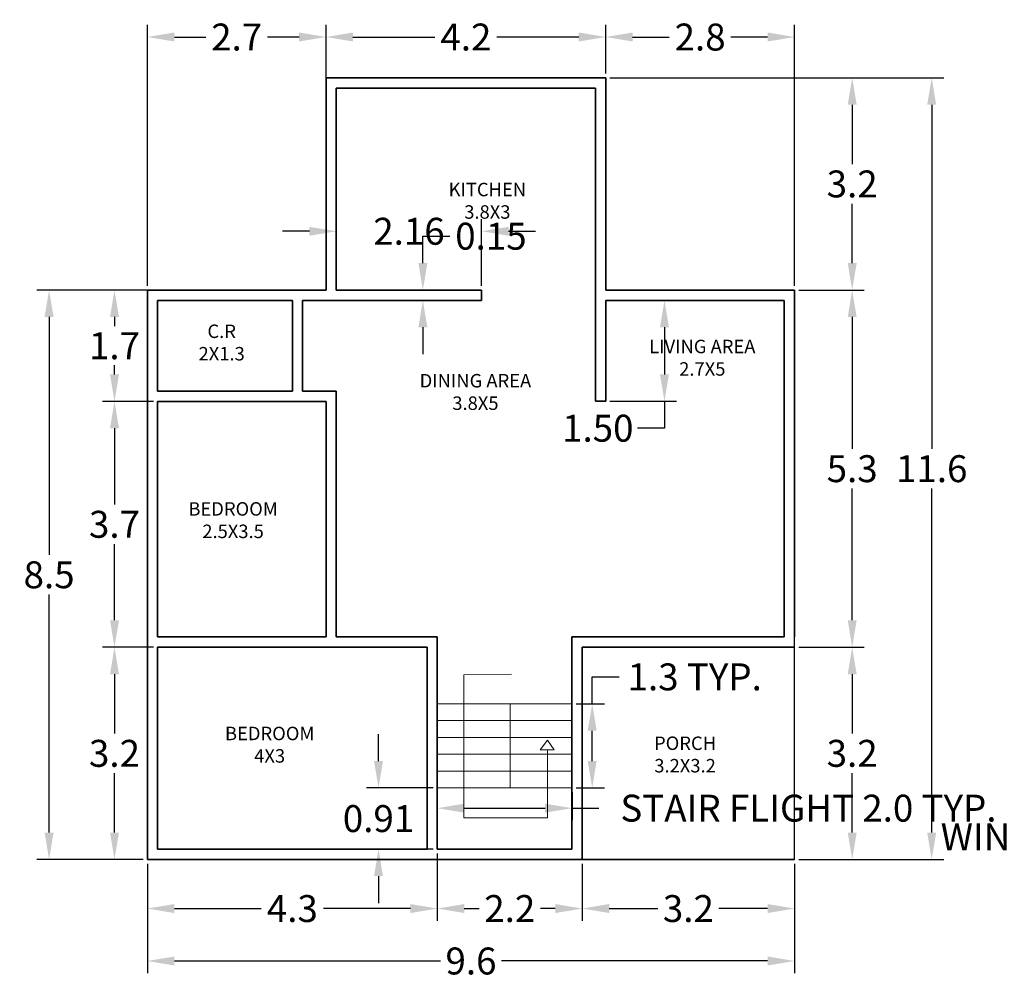
# Model space of a CAD drawing. Units: metres. Extents: x 24.2 to 58.5, y -14.5 to 15.2.
# Tile 2 of 7: x 24.2 to 38.9, y 0.1 to 14.4. Entities that reach past the tile are written whole.
import ezdxf

# ---------------------------------------------------------------- set-up
doc = ezdxf.new("R2010")
doc.units = ezdxf.units.M
doc.header["$MEASUREMENT"] = 0
for name, color, linetype, lineweight in [('A-ANNO-SYMB', 90, 'Continuous', 18), ('A-AREA-IDEN', 1, 'Continuous', 18), ('A-FLOR', 7, 'Continuous', 25), ('A-FLOR-STRS', 7, 'Continuous', 18), ('A-WALL', 7, 'Continuous', 35), ('DIMENSION', 90, 'Continuous', 18)]:
    doc.layers.add(name, color=color, linetype=linetype, lineweight=lineweight)
doc.styles.get("Standard").update_dxf_attribs({"font": 'arial.ttf'})
doc.dimstyles.get("Standard").update_dxf_attribs({"dimtxt": 0.4, "dimasz": 0.4, "dimexe": 0.18, "dimexo": 0.0625, "dimgap": 0.09, "dimtad": 0, "dimtih": 1, "dimtoh": 1, "dimdec": 1, "dimzin": 0, "dimdsep": 46, "dimtxsty": 'Standard', "dimcen": 0.09, "dimadec": 0, "dimazin": 0, "dimtfac": 1, "dimtdec": 1, "dimtofl": 0, "dimtmove": 0, "dimatfit": 3, "dimfxl": 1, "dimtolj": 1, "dimtzin": 0, "dimarcsym": 0})

# ---------------------------------------------------------------- blocks, each defined once
blk = doc.blocks.new('*D1')
at = {"layer": 'Defpoints', "color": 0, "transparency": 16777216}
for p in [(30.434, 2.049), (26.129, 1.896), (30.434, 1.168)]:
    blk.add_point(p, dxfattribs=at)
at = {"layer": 'DIMENSION', "color": 0, "lineweight": -2, "transparency": 16777216}
for p, q in [((30.434, 1.986), (30.434, 0.988)), ((26.129, 1.834), (26.129, 0.988)), ((26.529, 1.168), (27.819, 1.168)), ((30.034, 1.168), (28.744, 1.168))]:
    blk.add_line(p, q, dxfattribs=at)
at = {"layer": 'DIMENSION', "color": 0, "transparency": 16777216}
for points in [[(26.529, 1.235), (26.529, 1.101), (26.129, 1.168)], [(30.034, 1.235), (30.034, 1.101), (30.434, 1.168)]]:
    blk.add_solid(points, dxfattribs=at)
at = {"layer": 'DIMENSION', "color": 0, "transparency": 16777216, "insert": (28.281, 1.168), "char_height": 0.4, "attachment_point": 5}
blk.add_mtext('\\A1;4.3', dxfattribs=at)
blk = doc.blocks.new('*D2')
at = {"layer": 'Defpoints', "color": 0, "transparency": 16777216}
for p in [(30.434, 2.049), (32.586, 1.896), (32.586, 1.168)]:
    blk.add_point(p, dxfattribs=at)
at = {"layer": 'DIMENSION', "color": 0, "lineweight": -2, "transparency": 16777216}
for p, q in [((30.434, 1.986), (30.434, 0.988)), ((32.586, 1.834), (32.586, 0.988)), ((30.834, 1.168), (31.054, 1.168)), ((32.186, 1.168), (31.965, 1.168))]:
    blk.add_line(p, q, dxfattribs=at)
at = {"layer": 'DIMENSION', "color": 0, "transparency": 16777216}
for points in [[(30.834, 1.235), (30.834, 1.101), (30.434, 1.168)], [(32.186, 1.235), (32.186, 1.101), (32.586, 1.168)]]:
    blk.add_solid(points, dxfattribs=at)
at = {"layer": 'DIMENSION', "color": 0, "transparency": 16777216, "insert": (31.51, 1.168), "char_height": 0.4, "attachment_point": 5}
blk.add_mtext('\\A1;2.2', dxfattribs=at)
blk = doc.blocks.new('*D3')
at = {"layer": 'Defpoints', "color": 0, "transparency": 16777216}
for p in [(32.586, 1.896), (35.739, 1.896), (35.739, 1.168)]:
    blk.add_point(p, dxfattribs=at)
at = {"layer": 'DIMENSION', "color": 0, "lineweight": -2, "transparency": 16777216}
for p, q in [((32.586, 1.834), (32.586, 0.988)), ((35.739, 1.834), (35.739, 0.988)), ((32.986, 1.168), (33.71, 1.168)), ((35.339, 1.168), (34.614, 1.168))]:
    blk.add_line(p, q, dxfattribs=at)
at = {"layer": 'DIMENSION', "color": 0, "transparency": 16777216}
for points in [[(32.986, 1.235), (32.986, 1.101), (32.586, 1.168)], [(35.339, 1.235), (35.339, 1.101), (35.739, 1.168)]]:
    blk.add_solid(points, dxfattribs=at)
at = {"layer": 'DIMENSION', "color": 0, "transparency": 16777216, "insert": (34.162, 1.168), "char_height": 0.4, "attachment_point": 5}
blk.add_mtext('\\A1;3.2', dxfattribs=at)
blk = doc.blocks.new('*D4')
at = {"layer": 'Defpoints', "color": 0, "transparency": 16777216}
for p in [(25.64, 5.049), (26.281, 5.049), (26.129, 1.896)]:
    blk.add_point(p, dxfattribs=at)
at = {"layer": 'DIMENSION', "color": 0, "lineweight": -2, "transparency": 16777216}
for p, q in [((26.219, 5.049), (25.46, 5.049)), ((25.64, 4.649), (25.64, 3.767)), ((25.64, 2.296), (25.64, 3.178)), ((26.066, 1.896), (25.46, 1.896))]:
    blk.add_line(p, q, dxfattribs=at)
at = {"layer": 'DIMENSION', "color": 0, "transparency": 16777216}
for points in [[(25.574, 4.649), (25.707, 4.649), (25.64, 5.049)], [(25.574, 2.296), (25.707, 2.296), (25.64, 1.896)]]:
    blk.add_solid(points, dxfattribs=at)
at = {"layer": 'DIMENSION', "color": 0, "transparency": 16777216, "insert": (25.64, 3.473), "char_height": 0.4, "attachment_point": 5}
blk.add_mtext('\\A1;3.2', dxfattribs=at)
blk = doc.blocks.new('*D5')
at = {"layer": 'Defpoints', "color": 0, "transparency": 16777216}
for p in [(25.64, 8.701), (26.281, 8.701), (26.281, 5.049)]:
    blk.add_point(p, dxfattribs=at)
at = {"layer": 'DIMENSION', "color": 0, "lineweight": -2, "transparency": 16777216}
for p, q in [((26.219, 8.701), (25.46, 8.701)), ((25.64, 8.301), (25.64, 7.169)), ((25.64, 5.449), (25.64, 6.581)), ((26.219, 5.049), (25.46, 5.049))]:
    blk.add_line(p, q, dxfattribs=at)
at = {"layer": 'DIMENSION', "color": 0, "transparency": 16777216}
for points in [[(25.574, 8.301), (25.707, 8.301), (25.64, 8.701)], [(25.574, 5.449), (25.707, 5.449), (25.64, 5.049)]]:
    blk.add_solid(points, dxfattribs=at)
at = {"layer": 'DIMENSION', "color": 0, "transparency": 16777216, "insert": (25.64, 6.875), "char_height": 0.4, "attachment_point": 5}
blk.add_mtext('\\A1;3.7', dxfattribs=at)
blk = doc.blocks.new('*D6')
at = {"layer": 'Defpoints', "color": 0, "transparency": 16777216}
for p in [(25.64, 10.354), (26.281, 10.354), (26.281, 8.701)]:
    blk.add_point(p, dxfattribs=at)
at = {"layer": 'DIMENSION', "color": 0, "lineweight": -2, "transparency": 16777216}
for p, q in [((26.219, 10.354), (25.46, 10.354)), ((25.64, 9.954), (25.64, 9.818)), ((25.64, 9.101), (25.64, 9.237)), ((26.219, 8.701), (25.46, 8.701))]:
    blk.add_line(p, q, dxfattribs=at)
at = {"layer": 'DIMENSION', "color": 0, "transparency": 16777216}
for points in [[(25.574, 9.954), (25.707, 9.954), (25.64, 10.354)], [(25.574, 9.101), (25.707, 9.101), (25.64, 8.701)]]:
    blk.add_solid(points, dxfattribs=at)
at = {"layer": 'DIMENSION', "color": 0, "transparency": 16777216, "insert": (25.64, 9.527), "char_height": 0.4, "attachment_point": 5}
blk.add_mtext('\\A1;1.7', dxfattribs=at)
blk = doc.blocks.new('*D7')
at = {"layer": 'Defpoints', "color": 0, "transparency": 16777216}
for p in [(28.781, 14.112), (26.129, 10.354), (28.781, 10.354)]:
    blk.add_point(p, dxfattribs=at)
at = {"layer": 'DIMENSION', "color": 0, "lineweight": -2, "transparency": 16777216}
for p, q in [((26.129, 10.416), (26.129, 14.292)), ((28.781, 10.416), (28.781, 14.292)), ((26.529, 14.112), (26.998, 14.112)), ((28.381, 14.112), (27.913, 14.112))]:
    blk.add_line(p, q, dxfattribs=at)
at = {"layer": 'DIMENSION', "color": 0, "transparency": 16777216}
for points in [[(26.529, 14.179), (26.529, 14.046), (26.129, 14.112)], [(28.381, 14.179), (28.381, 14.046), (28.781, 14.112)]]:
    blk.add_solid(points, dxfattribs=at)
at = {"layer": 'DIMENSION', "color": 0, "transparency": 16777216, "insert": (27.455, 14.112), "char_height": 0.4, "attachment_point": 5}
blk.add_mtext('\\A1;2.7', dxfattribs=at)
blk = doc.blocks.new('*D8')
at = {"layer": 'Defpoints', "color": 0, "transparency": 16777216}
for p in [(32.934, 14.112), (32.934, 13.506), (28.781, 10.354)]:
    blk.add_point(p, dxfattribs=at)
at = {"layer": 'DIMENSION', "color": 0, "lineweight": -2, "transparency": 16777216}
for p, q in [((28.781, 10.416), (28.781, 14.292)), ((32.934, 13.569), (32.934, 14.292)), ((29.181, 14.112), (30.397, 14.112)), ((32.534, 14.112), (31.318, 14.112))]:
    blk.add_line(p, q, dxfattribs=at)
at = {"layer": 'DIMENSION', "color": 0, "transparency": 16777216}
for points in [[(29.181, 14.179), (29.181, 14.046), (28.781, 14.112)], [(32.534, 14.179), (32.534, 14.046), (32.934, 14.112)]]:
    blk.add_solid(points, dxfattribs=at)
at = {"layer": 'DIMENSION', "color": 0, "transparency": 16777216, "insert": (30.858, 14.112), "char_height": 0.4, "attachment_point": 5}
blk.add_mtext('\\A1;4.2', dxfattribs=at)
blk = doc.blocks.new('*D9')
at = {"layer": 'Defpoints', "color": 0, "transparency": 16777216}
for p in [(35.739, 14.112), (32.934, 13.506), (35.739, 10.354)]:
    blk.add_point(p, dxfattribs=at)
at = {"layer": 'DIMENSION', "color": 0, "lineweight": -2, "transparency": 16777216}
for p, q in [((32.934, 13.569), (32.934, 14.292)), ((35.739, 10.416), (35.739, 14.292)), ((33.334, 14.112), (33.878, 14.112)), ((35.339, 14.112), (34.794, 14.112))]:
    blk.add_line(p, q, dxfattribs=at)
at = {"layer": 'DIMENSION', "color": 0, "transparency": 16777216}
for points in [[(33.334, 14.179), (33.334, 14.046), (32.934, 14.112)], [(35.339, 14.179), (35.339, 14.046), (35.739, 14.112)]]:
    blk.add_solid(points, dxfattribs=at)
at = {"layer": 'DIMENSION', "color": 0, "transparency": 16777216, "insert": (34.336, 14.112), "char_height": 0.4, "attachment_point": 5}
blk.add_mtext('\\A1;2.8', dxfattribs=at)
blk = doc.blocks.new('*D10')
at = {"layer": 'Defpoints', "color": 0, "transparency": 16777216}
for p in [(35.739, 5.049), (36.594, 5.049), (35.739, 1.896)]:
    blk.add_point(p, dxfattribs=at)
at = {"layer": 'DIMENSION', "color": 0, "lineweight": -2, "transparency": 16777216}
for p, q in [((35.801, 5.049), (36.774, 5.049)), ((36.594, 4.649), (36.594, 3.767)), ((36.594, 2.296), (36.594, 3.178)), ((35.801, 1.896), (36.774, 1.896))]:
    blk.add_line(p, q, dxfattribs=at)
at = {"layer": 'DIMENSION', "color": 0, "transparency": 16777216}
for points in [[(36.528, 4.649), (36.661, 4.649), (36.594, 5.049)], [(36.528, 2.296), (36.661, 2.296), (36.594, 1.896)]]:
    blk.add_solid(points, dxfattribs=at)
at = {"layer": 'DIMENSION', "color": 0, "transparency": 16777216, "insert": (36.594, 3.473), "char_height": 0.4, "attachment_point": 5}
blk.add_mtext('\\A1;3.2', dxfattribs=at)
blk = doc.blocks.new('*D11')
at = {"layer": 'Defpoints', "color": 0, "transparency": 16777216}
for p in [(35.739, 10.354), (36.594, 10.354), (35.739, 5.049)]:
    blk.add_point(p, dxfattribs=at)
at = {"layer": 'DIMENSION', "color": 0, "lineweight": -2, "transparency": 16777216}
for p, q in [((35.801, 10.354), (36.774, 10.354)), ((36.594, 9.954), (36.594, 7.996)), ((36.594, 5.449), (36.594, 7.407)), ((35.801, 5.049), (36.774, 5.049))]:
    blk.add_line(p, q, dxfattribs=at)
at = {"layer": 'DIMENSION', "color": 0, "transparency": 16777216}
for points in [[(36.528, 9.954), (36.661, 9.954), (36.594, 10.354)], [(36.528, 5.449), (36.661, 5.449), (36.594, 5.049)]]:
    blk.add_solid(points, dxfattribs=at)
at = {"layer": 'DIMENSION', "color": 0, "transparency": 16777216, "insert": (36.594, 7.701), "char_height": 0.4, "attachment_point": 5}
blk.add_mtext('\\A1;5.3', dxfattribs=at)
blk = doc.blocks.new('*D12')
at = {"layer": 'Defpoints', "color": 0, "transparency": 16777216}
for p in [(32.934, 13.506), (36.594, 13.506), (35.739, 10.354)]:
    blk.add_point(p, dxfattribs=at)
at = {"layer": 'DIMENSION', "color": 0, "lineweight": -2, "transparency": 16777216}
for p, q in [((32.996, 13.506), (36.774, 13.506)), ((36.594, 13.106), (36.594, 12.224)), ((36.594, 10.754), (36.594, 11.635)), ((35.801, 10.354), (36.774, 10.354))]:
    blk.add_line(p, q, dxfattribs=at)
at = {"layer": 'DIMENSION', "color": 0, "transparency": 16777216}
for points in [[(36.528, 13.106), (36.661, 13.106), (36.594, 13.506)], [(36.528, 10.754), (36.661, 10.754), (36.594, 10.354)]]:
    blk.add_solid(points, dxfattribs=at)
at = {"layer": 'DIMENSION', "color": 0, "transparency": 16777216, "insert": (36.594, 11.93), "char_height": 0.4, "attachment_point": 5}
blk.add_mtext('\\A1;3.2', dxfattribs=at)
blk = doc.blocks.new('*D13')
at = {"layer": 'Defpoints', "color": 0, "transparency": 16777216}
for p in [(35.739, 13.506), (37.775, 13.506), (35.739, 1.896)]:
    blk.add_point(p, dxfattribs=at)
at = {"layer": 'DIMENSION', "color": 0, "lineweight": -2, "transparency": 16777216}
for p, q in [((35.801, 13.506), (37.955, 13.506)), ((37.775, 13.106), (37.775, 7.995)), ((37.775, 2.296), (37.775, 7.407)), ((35.801, 1.896), (37.955, 1.896))]:
    blk.add_line(p, q, dxfattribs=at)
at = {"layer": 'DIMENSION', "color": 0, "transparency": 16777216}
for points in [[(37.708, 13.106), (37.841, 13.106), (37.775, 13.506)], [(37.708, 2.296), (37.841, 2.296), (37.775, 1.896)]]:
    blk.add_solid(points, dxfattribs=at)
at = {"layer": 'DIMENSION', "color": 0, "transparency": 16777216, "insert": (37.775, 7.701), "char_height": 0.4, "attachment_point": 5}
blk.add_mtext('\\A1;11.6', dxfattribs=at)
blk = doc.blocks.new('*D14')
at = {"layer": 'Defpoints', "color": 0, "transparency": 16777216}
for p in [(26.129, 1.896), (35.739, 1.896), (35.739, 0.389)]:
    blk.add_point(p, dxfattribs=at)
at = {"layer": 'DIMENSION', "color": 0, "lineweight": -2, "transparency": 16777216}
for p, q in [((26.129, 1.834), (26.129, 0.209)), ((35.739, 1.834), (35.739, 0.209)), ((26.529, 0.389), (30.48, 0.389)), ((35.339, 0.389), (31.388, 0.389))]:
    blk.add_line(p, q, dxfattribs=at)
at = {"layer": 'DIMENSION', "color": 0, "transparency": 16777216}
for points in [[(26.529, 0.456), (26.529, 0.322), (26.129, 0.389)], [(35.339, 0.456), (35.339, 0.322), (35.739, 0.389)]]:
    blk.add_solid(points, dxfattribs=at)
at = {"layer": 'DIMENSION', "color": 0, "transparency": 16777216, "insert": (30.934, 0.389), "char_height": 0.4, "attachment_point": 5}
blk.add_mtext('\\A1;9.6', dxfattribs=at)
blk = doc.blocks.new('*D15')
at = {"layer": 'Defpoints', "color": 0, "transparency": 16777216}
for p in [(24.669, 10.354), (26.129, 10.354), (26.129, 1.896)]:
    blk.add_point(p, dxfattribs=at)
at = {"layer": 'DIMENSION', "color": 0, "lineweight": -2, "transparency": 16777216}
for p, q in [((26.066, 10.354), (24.489, 10.354)), ((24.669, 9.954), (24.669, 6.419)), ((24.669, 2.296), (24.669, 5.831)), ((26.066, 1.896), (24.489, 1.896))]:
    blk.add_line(p, q, dxfattribs=at)
at = {"layer": 'DIMENSION', "color": 0, "transparency": 16777216}
for points in [[(24.602, 9.954), (24.736, 9.954), (24.669, 10.354)], [(24.602, 2.296), (24.736, 2.296), (24.669, 1.896)]]:
    blk.add_solid(points, dxfattribs=at)
at = {"layer": 'DIMENSION', "color": 0, "transparency": 16777216, "insert": (24.669, 6.125), "char_height": 0.4, "attachment_point": 5}
blk.add_mtext('\\A1;8.5', dxfattribs=at)
blk = doc.blocks.new('STAIR-FLIGHT-2000')
for p, q in [((0, 1.25), (2, 1.25)), ((0, 1), (2, 1)), ((0, 0.75), (2, 0.75)), ((0, 0.5), (2, 0.5)), ((0, 0.25), (2, 0.25)), ((0, 0), (2, 0))]:
    blk.add_line(p, q)
blk = doc.blocks.new('STAIR-PATH-UP')
for p, q in [((0.708, 2.134), (0, 2.121)), ((0, 2.121), (0, 0)), ((1.133, 1.007), (1.242, 1.15)), ((1.242, 1.15), (1.342, 1.007)), ((1.242, 1.007), (1.133, 1.007)), ((1.242, 0), (1.242, 1.007)), ((1.342, 1.007), (1.242, 1.007)), ((0, 0), (1.242, 0))]:
    blk.add_line(p, q)
blk = doc.blocks.new('*D61')
at = {"layer": 'Defpoints', "color": 0, "transparency": 16777216}
for p in [(42.965, 2.232), (42.965, 2.049), (44.185, 2.049)]:
    blk.add_point(p, dxfattribs=at)
at = {"layer": 'DIMENSION', "color": 0, "lineweight": -2, "transparency": 16777216}
for p, q in [((42.965, 2.111), (42.965, 2.412)), ((44.185, 2.111), (44.185, 2.412)), ((42.965, 2.232), (42.565, 2.232)), ((43.785, 2.232), (43.365, 2.232))]:
    blk.add_line(p, q, dxfattribs=at)
at = {"layer": 'DIMENSION', "color": 0, "transparency": 16777216}
for points in [[(43.365, 2.298), (43.365, 2.165), (42.965, 2.232)], [(43.785, 2.298), (43.785, 2.165), (44.185, 2.232)]]:
    blk.add_solid(points, dxfattribs=at)
at = {"layer": 'DIMENSION', "color": 0, "transparency": 16777216, "insert": (40.113, 2.232), "char_height": 0.4, "attachment_point": 5}
blk.add_mtext('\\A1;WINDOW 1.2 TYP.', dxfattribs=at)
blk = doc.blocks.new('*D65')
at = {"layer": 'Defpoints', "color": 0, "transparency": 16777216}
for p in [(30.434, 2.959), (32.434, 2.959), (32.434, 2.659)]:
    blk.add_point(p, dxfattribs=at)
at = {"layer": 'DIMENSION', "color": 0, "lineweight": -2, "transparency": 16777216}
for p, q in [((30.434, 2.896), (30.434, 2.479)), ((32.434, 2.896), (32.434, 2.479)), ((30.834, 2.659), (32.034, 2.659)), ((32.434, 2.659), (32.834, 2.659))]:
    blk.add_line(p, q, dxfattribs=at)
at = {"layer": 'DIMENSION', "color": 0, "transparency": 16777216}
for points in [[(30.834, 2.725), (30.834, 2.592), (30.434, 2.659)], [(32.034, 2.725), (32.034, 2.592), (32.434, 2.659)]]:
    blk.add_solid(points, dxfattribs=at)
at = {"layer": 'DIMENSION', "color": 0, "transparency": 16777216, "insert": (35.945, 2.659), "char_height": 0.4, "attachment_point": 5}
blk.add_mtext('\\A1;STAIR FLIGHT 2.0 TYP.', dxfattribs=at)
blk = doc.blocks.new('*D66')
at = {"layer": 'Defpoints', "color": 0, "transparency": 16777216}
for p in [(32.434, 4.209), (32.734, 4.209), (32.434, 2.959)]:
    blk.add_point(p, dxfattribs=at)
at = {"layer": 'DIMENSION', "color": 0, "lineweight": -2, "transparency": 16777216}
for p, q in [((32.734, 4.209), (32.734, 4.609)), ((32.734, 4.609), (33.134, 4.609)), ((32.496, 4.209), (32.914, 4.209)), ((32.734, 3.359), (32.734, 3.809)), ((32.496, 2.959), (32.914, 2.959))]:
    blk.add_line(p, q, dxfattribs=at)
at = {"layer": 'DIMENSION', "color": 0, "transparency": 16777216}
for points in [[(32.667, 3.809), (32.8, 3.809), (32.734, 4.209)], [(32.667, 3.359), (32.8, 3.359), (32.734, 2.959)]]:
    blk.add_solid(points, dxfattribs=at)
at = {"layer": 'DIMENSION', "color": 0, "transparency": 16777216, "insert": (34.256, 4.609), "char_height": 0.4, "attachment_point": 5}
blk.add_mtext('\\A1;1.3 TYP.', dxfattribs=at)
blk = doc.blocks.new('*D103')
at = {"layer": 'Defpoints', "color": 0, "transparency": 16777216}
for p in [(31.092, 11.227), (28.934, 10.354), (31.092, 10.354)]:
    blk.add_point(p, dxfattribs=at)
at = {"layer": 'DIMENSION', "color": 0, "lineweight": -2, "transparency": 16777216}
for p, q in [((28.934, 10.416), (28.934, 11.407)), ((31.092, 10.416), (31.092, 11.407)), ((28.534, 11.227), (28.134, 11.227)), ((31.492, 11.227), (31.892, 11.227))]:
    blk.add_line(p, q, dxfattribs=at)
at = {"layer": 'DIMENSION', "color": 0, "transparency": 16777216}
for points in [[(28.534, 11.293), (28.534, 11.16), (28.934, 11.227)], [(31.492, 11.293), (31.492, 11.16), (31.092, 11.227)]]:
    blk.add_solid(points, dxfattribs=at)
at = {"layer": 'DIMENSION', "color": 0, "transparency": 16777216, "insert": (30.013, 11.227), "char_height": 0.4, "attachment_point": 5}
blk.add_mtext('\\A1;2.16', dxfattribs=at)
blk = doc.blocks.new('*D104')
at = {"layer": 'Defpoints', "color": 0, "transparency": 16777216}
for p in [(32.934, 10.201), (32.934, 8.702), (33.807, 8.702)]:
    blk.add_point(p, dxfattribs=at)
at = {"layer": 'DIMENSION', "color": 0, "lineweight": -2, "transparency": 16777216}
for p, q in [((32.996, 10.201), (33.987, 10.201)), ((33.807, 9.801), (33.807, 9.102)), ((32.996, 8.702), (33.987, 8.702)), ((33.807, 8.702), (33.807, 8.302)), ((33.807, 8.302), (33.407, 8.302))]:
    blk.add_line(p, q, dxfattribs=at)
at = {"layer": 'DIMENSION', "color": 0, "transparency": 16777216}
for points in [[(33.74, 9.801), (33.873, 9.801), (33.807, 10.201)], [(33.74, 9.102), (33.873, 9.102), (33.807, 8.702)]]:
    blk.add_solid(points, dxfattribs=at)
at = {"layer": 'DIMENSION', "color": 0, "transparency": 16777216, "insert": (32.817, 8.302), "char_height": 0.4, "attachment_point": 5}
blk.add_mtext('\\A1;1.50', dxfattribs=at)
blk = doc.blocks.new('*D105')
at = {"layer": 'Defpoints', "color": 0, "transparency": 16777216}
for p in [(30.219, 10.354), (31.092, 10.354), (31.092, 10.201)]:
    blk.add_point(p, dxfattribs=at)
at = {"layer": 'DIMENSION', "color": 0, "lineweight": -2, "transparency": 16777216}
for p, q in [((30.219, 10.754), (30.219, 11.154)), ((30.219, 11.154), (30.619, 11.154)), ((31.03, 10.354), (30.039, 10.354)), ((31.03, 10.201), (30.039, 10.201)), ((30.219, 9.801), (30.219, 9.401))]:
    blk.add_line(p, q, dxfattribs=at)
at = {"layer": 'DIMENSION', "color": 0, "transparency": 16777216}
for points in [[(30.153, 10.754), (30.286, 10.754), (30.219, 10.354)], [(30.153, 9.801), (30.286, 9.801), (30.219, 10.201)]]:
    blk.add_solid(points, dxfattribs=at)
at = {"layer": 'DIMENSION', "color": 0, "transparency": 16777216, "insert": (31.23, 11.154), "char_height": 0.4, "attachment_point": 5}
blk.add_mtext('\\A1;0.15', dxfattribs=at)
blk = doc.blocks.new('*D106')
at = {"layer": 'Defpoints', "color": 0, "transparency": 16777216}
for p in [(29.561, 2.959), (30.434, 2.959), (30.434, 2.049)]:
    blk.add_point(p, dxfattribs=at)
at = {"layer": 'DIMENSION', "color": 0, "lineweight": -2, "transparency": 16777216}
for p, q in [((29.561, 3.359), (29.561, 3.759)), ((30.371, 2.959), (29.381, 2.959)), ((30.371, 2.049), (29.381, 2.049)), ((29.561, 1.649), (29.561, 1.249))]:
    blk.add_line(p, q, dxfattribs=at)
at = {"layer": 'DIMENSION', "color": 0, "transparency": 16777216}
for points in [[(29.494, 3.359), (29.627, 3.359), (29.561, 2.959)], [(29.494, 1.649), (29.627, 1.649), (29.561, 2.049)]]:
    blk.add_solid(points, dxfattribs=at)
at = {"layer": 'DIMENSION', "color": 0, "transparency": 16777216, "insert": (29.561, 2.504), "char_height": 0.4, "attachment_point": 5}
blk.add_mtext('\\A1;0.91', dxfattribs=at)

msp = doc.modelspace()

# ---------------------------------------------------------------- linework, layer by layer
at = {"layer": 'A-FLOR'}
msp.add_line((35.7385, 1.8964), (35.7385, 5.2012), dxfattribs=at)
at = {"layer": 'A-FLOR-STRS'}
msp.add_line((31.5141, 2.9588), (31.5141, 4.2088), dxfattribs=at)
at = {"layer": 'A-WALL'}
for p, q in [((28.7813, 13.506), (32.9337, 13.506)), ((28.7813, 10.3536), (28.7813, 13.506)), ((32.9337, 10.3536), (32.9337, 13.506)), ((28.9337, 13.3536), (32.7813, 13.3536)), ((28.9337, 10.3536), (28.9337, 13.3536)), ((32.7813, 8.7016), (32.7813, 13.3536)), ((26.1289, 1.8964), (26.1289, 10.3536)), ((26.1289, 10.3536), (28.7813, 10.3536)), ((28.9337, 10.3536), (31.0923, 10.3536)), ((31.0923, 10.2012), (31.0923, 10.3536)), ((32.9337, 10.3536), (35.7385, 10.3536)), ((35.7385, 5.2012), (35.7385, 10.3536)), ((26.2813, 10.2012), (28.2813, 10.2012)), ((26.2813, 8.8536), (26.2813, 10.2012)), ((28.2813, 8.8536), (28.2813, 10.2012)), ((28.4337, 10.2012), (31.0923, 10.2012)), ((28.4337, 8.8536), (28.4337, 10.2012)), ((32.9337, 10.2012), (32.9337, 8.7016)), ((32.9337, 10.2012), (35.5861, 10.2012)), ((35.5861, 5.2012), (35.5861, 10.2012)), ((26.2813, 8.8536), (28.2813, 8.8536)), ((28.4337, 8.8536), (28.9337, 8.8536)), ((28.9337, 5.2012), (28.9337, 8.8536)), ((26.2813, 5.2012), (26.2813, 8.7012)), ((26.2813, 8.7012), (28.7813, 8.7012)), ((28.7813, 5.2012), (28.7813, 8.7012)), ((32.7813, 8.7016), (32.9337, 8.7016)), ((26.2813, 5.2012), (28.7813, 5.2012)), ((28.9337, 5.2012), (30.4337, 5.2012)), ((30.4337, 2.0488), (30.4337, 5.2012)), ((32.4337, 2.0488), (32.4337, 5.2012)), ((32.4337, 5.2012), (35.5861, 5.2012)), ((26.2813, 2.0488), (26.2813, 5.0488)), ((26.2813, 5.0488), (30.2813, 5.0488)), ((30.2813, 2.0488), (30.2813, 5.0488)), ((32.5861, 1.8964), (32.5861, 5.0488)), ((32.5861, 5.0488), (35.7385, 5.0488)), ((26.2813, 2.0488), (30.2813, 2.0488)), ((30.4337, 2.0488), (32.4337, 2.0488)), ((26.1289, 1.8964), (35.7385, 1.8964))]:
    msp.add_line(p, q, dxfattribs=at)

# ---------------------------------------------------------------- block references
at = {"layer": 'A-ANNO-SYMB'}
msp.add_blockref('STAIR-PATH-UP', (30.826, 2.517), dxfattribs=at)
at = {"layer": 'A-FLOR-STRS'}
msp.add_blockref('STAIR-FLIGHT-2000', (30.434, 2.959), dxfattribs=at)

# ---------------------------------------------------------------- texts
at = {"layer": 'A-AREA-IDEN', "char_height": 0.2, "attachment_point": 2}
for s, width, insert in [('KITCHEN\\P3.8X3', 1.744906, (31.177, 11.9469)), ('C.R\\P2X1.3', 1.744906, (27.2317, 9.8419)), ('LIVING AREA\\P2.7X5', 3.418042, (34.369, 9.6158)), ('DINING AREA\\P3.8X5', 2.961404, (30.9999, 9.1072)), ('BEDROOM\\P2.5X3.5', 1.744906, (27.401, 7.2036)), ('BEDROOM\\P4X3', 1.744906, (27.9444, 3.8683)), ('PORCH\\P3.2X3.2', 1.744906, (34.1126, 3.7231))]:
    msp.add_mtext_dynamic_manual_height_columns(s, width=width, gutter_width=1, heights=[0], dxfattribs=dict(at, insert=insert))

# ---------------------------------------------------------------- dimensions: what is measured, and where the dimension line sits
at = {"layer": 'DIMENSION'}
for base, p1, p2, override, picture, middle in [((28.7813, 14.1124), (26.1289, 10.3536), (28.7813, 10.3536), {"dimclrd": 0, "dimclre": 0, "dimclrt": 0}, '*D7', (27.4551, 14.1124)), ((32.9337, 14.1124), (28.7813, 10.3536), (32.9337, 13.506), {"dimclrd": 0, "dimclre": 0, "dimclrt": 0, "dimtmove": 1}, '*D8', (30.8575, 14.1124)), ((35.7385, 14.1124), (32.9337, 13.506), (35.7385, 10.3536), {"dimclrd": 0, "dimclre": 0, "dimclrt": 0, "dimtmove": 1}, '*D9', (34.3361, 14.1124)), ((30.4337, 1.168), (26.1289, 1.8964), (30.4337, 2.0488), {"dimclrd": 0, "dimclre": 0, "dimclrt": 0}, '*D1', (28.2813, 1.168)), ((32.5861, 1.168), (30.4337, 2.0488), (32.5861, 1.8964), {"dimclrd": 0, "dimclre": 0, "dimclrt": 0, "dimtmove": 1}, '*D2', (31.5099, 1.168)), ((35.7385, 0.3889), (26.1289, 1.8964), (35.7385, 1.8964), {"dimclrd": 0, "dimclre": 0, "dimclrt": 0}, '*D14', (30.9337, 0.3889)), ((35.7385, 1.168), (32.5861, 1.8964), (35.7385, 1.8964), {"dimclrd": 0, "dimclre": 0, "dimclrt": 0, "dimtmove": 1}, '*D3', (34.1623, 1.168))]:
    dim = msp.add_linear_dim(base=base, p1=p1, p2=p2, dimstyle='Standard', override=override, dxfattribs=at)
    dim.commit()
    dim.dimension.update_dxf_attribs({"geometry": picture, "text_midpoint": middle})
for base, p1, p2, angle, override, picture, middle in [((36.5945, 13.506), (35.7385, 10.3536), (32.9337, 13.506), 90, {"dimclrd": 0, "dimclre": 0, "dimclrt": 0, "dimtmove": 1}, '*D12', (36.5945, 11.9298)), ((37.7746, 13.506), (35.7385, 1.8964), (35.7385, 13.506), 90, {"dimclrd": 0, "dimclre": 0, "dimclrt": 0}, '*D13', (37.7746, 7.7012)), ((31.0923, 11.2266), (28.9337, 10.3536), (31.0923, 10.3536), 0, {"dimdec": 2, "dimlfac": 1, "dimrnd": 0, "dimzin": 0, "dimdsep": 46, "dimlunit": 2}, '*D103', (30.013, 11.2266)), ((30.2193, 10.3536), (31.0923, 10.2012), (31.0923, 10.3536), 90, {"dimdec": 2, "dimlfac": 1, "dimrnd": 0, "dimzin": 0, "dimdsep": 46, "dimlunit": 2}, '*D105', (31.2303, 11.1536)), ((24.6689, 10.3536), (26.1289, 1.8964), (26.1289, 10.3536), 90, {"dimclrd": 0, "dimclre": 0, "dimclrt": 0}, '*D15', (24.6689, 6.125)), ((25.6402, 10.3536), (26.2813, 8.7012), (26.2813, 10.3536), 90, {"dimclrd": 0, "dimclre": 0, "dimclrt": 0, "dimtmove": 1}, '*D6', (25.6402, 9.5274)), ((36.5945, 10.3536), (35.7385, 5.0488), (35.7385, 10.3536), 90, {"dimclrd": 0, "dimclre": 0, "dimclrt": 0, "dimtmove": 1}, '*D11', (36.5945, 7.7012)), ((33.8067, 8.7016), (32.9337, 10.2012), (32.9337, 8.7016), 270, {"dimdec": 2, "dimlfac": 1, "dimrnd": 0, "dimzin": 0, "dimdsep": 46, "dimlunit": 2}, '*D104', (32.8167, 8.3016)), ((25.6402, 8.7012), (26.2813, 5.0488), (26.2813, 8.7012), 90, {"dimclrd": 0, "dimclre": 0, "dimclrt": 0, "dimtmove": 1}, '*D5', (25.6402, 6.875)), ((25.6402, 5.0488), (26.1289, 1.8964), (26.2813, 5.0488), 90, {"dimclrd": 0, "dimclre": 0, "dimclrt": 0}, '*D4', (25.6402, 3.4726)), ((36.5945, 5.0488), (35.7385, 1.8964), (35.7385, 5.0488), 90, {"dimclrd": 0, "dimclre": 0, "dimclrt": 0}, '*D10', (36.5945, 3.4726)), ((29.5607, 2.9588), (30.4337, 2.0488), (30.4337, 2.9588), 90, {"dimdec": 2, "dimlfac": 1, "dimrnd": 0, "dimzin": 0, "dimdsep": 46, "dimlunit": 2}, '*D106', (29.5607, 2.5038))]:
    dim = msp.add_linear_dim(base=base, p1=p1, p2=p2, angle=angle, dimstyle='Standard', override=override, dxfattribs=at)
    dim.commit()
    dim.dimension.update_dxf_attribs({"geometry": picture, "text_midpoint": middle})
for base, p1, p2, angle, text, picture, middle in [((32.7337450927, 4.2088239886), (32.4337450927, 2.9588239886), (32.4337450927, 4.2088239886), 90, '<> TYP.', '*D66', (34.2560779713, 4.6088239886)), ((42.9655, 2.2318), (44.1855, 2.0488), (42.9655, 2.0488), 180, 'WINDOW <> TYP.', '*D61', (40.1126, 2.2318))]:
    dim = msp.add_linear_dim(base=base, p1=p1, p2=p2, angle=angle, text=text, dimstyle='Standard', override={"dimdec": 1, "dimlfac": 1, "dimrnd": 0, "dimzin": 0, "dimdsep": 46, "dimlunit": 2}, dxfattribs=at)
    dim.commit()
    dim.dimension.update_dxf_attribs({"geometry": picture, "text_midpoint": middle})
dim = msp.add_linear_dim(base=(32.4337, 2.6588), p1=(30.4337, 2.9588), p2=(32.4337, 2.9588), text='STAIR FLIGHT <> TYP.', dimstyle='Standard', override={"dimdec": 1, "dimlfac": 1, "dimrnd": 0, "dimzin": 0, "dimdsep": 46, "dimlunit": 2}, dxfattribs=at)
dim.commit()
dim.dimension.update_dxf_attribs({"geometry": '*D65', "text_midpoint": (35.9454, 2.6588)})

doc.saveas('drawing.dxf')
